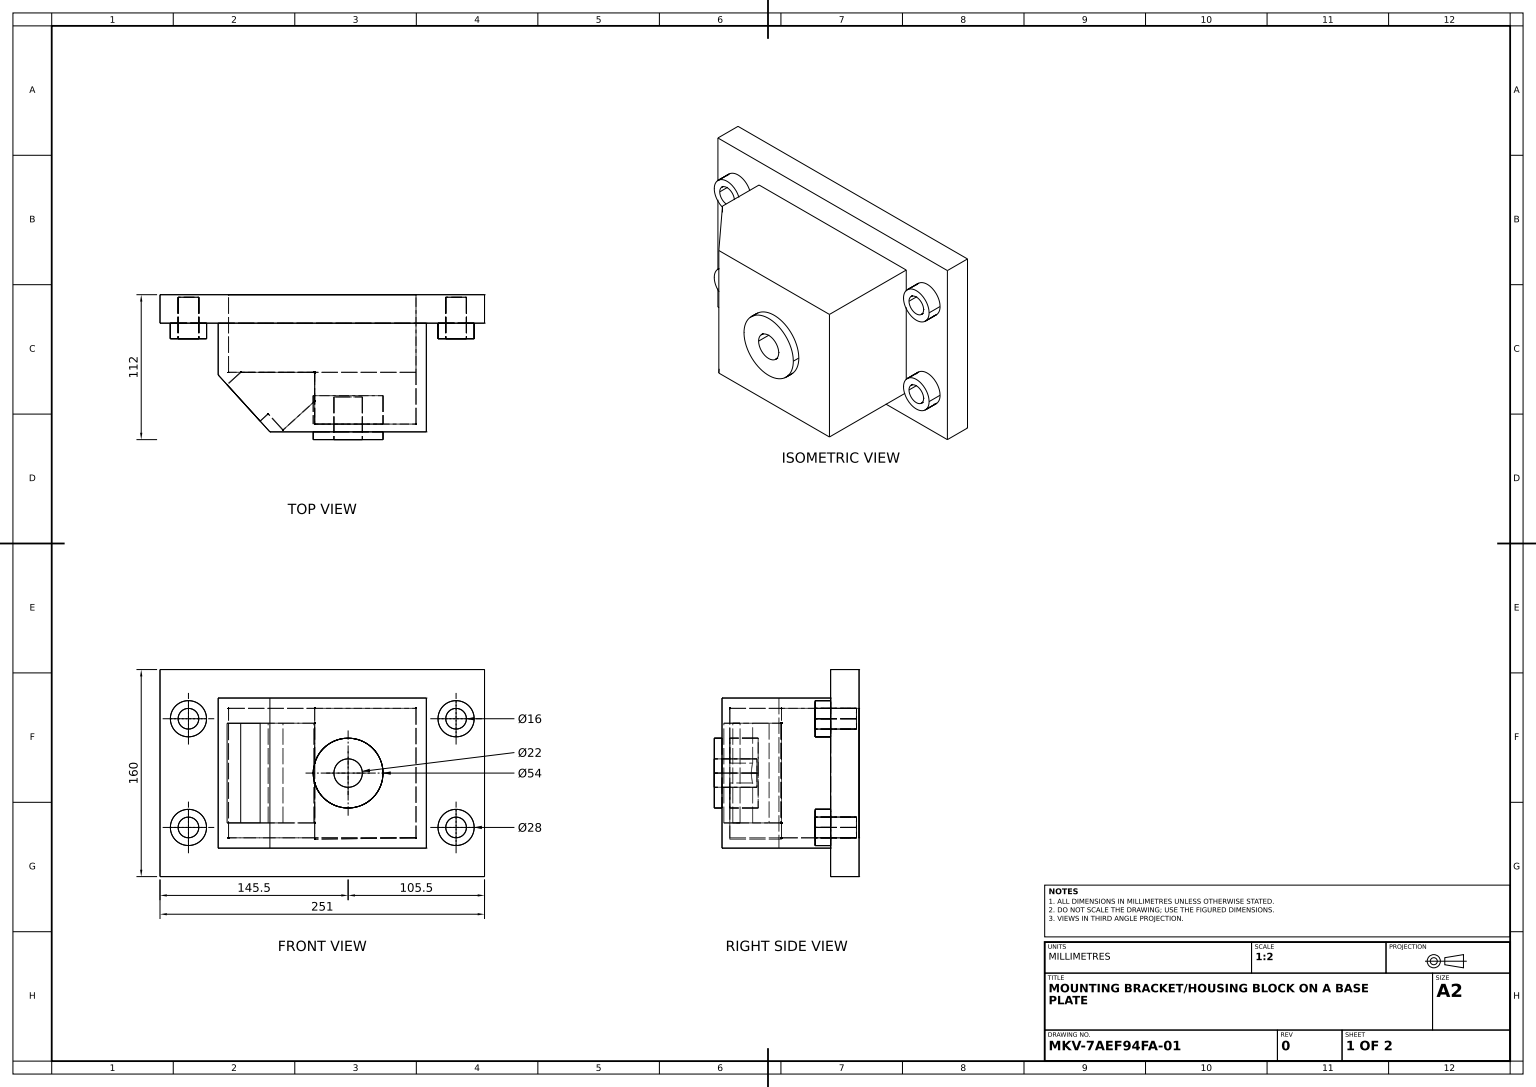
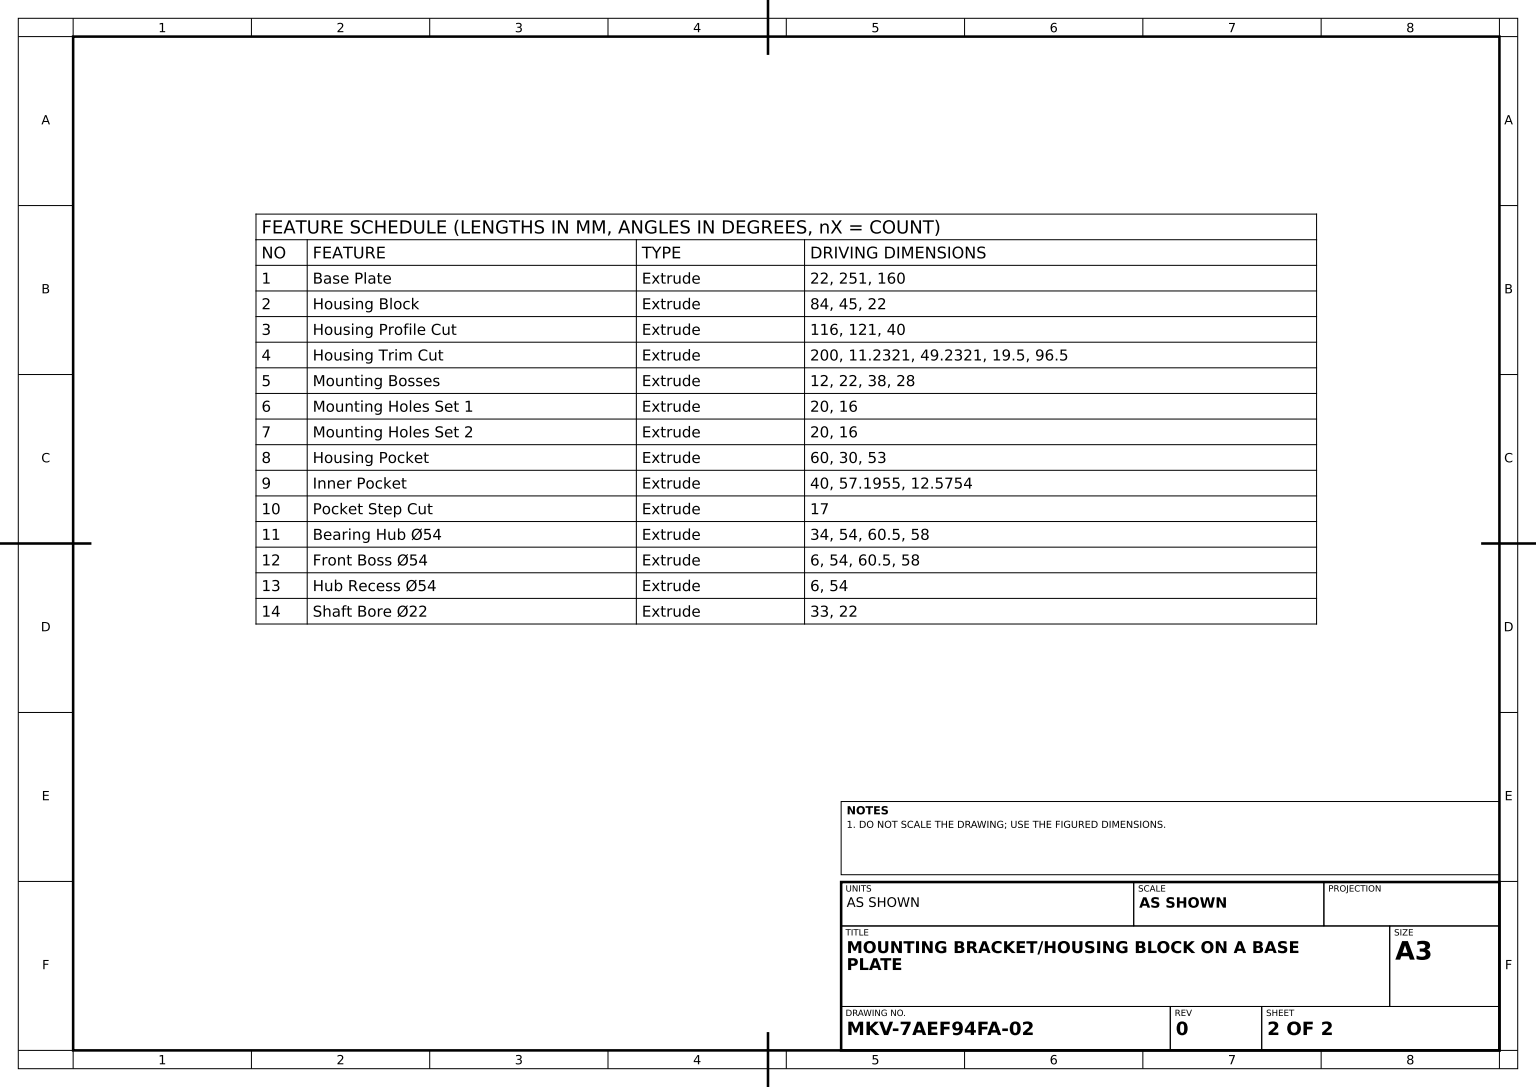
SolidWorks part; units mm, degrees
material "Plain Carbon Steel"
ref_plane "Front Plane" through (0, 0, 0) normal (0, 0, 1) x (1, 0, 0)
ref_plane "Top Plane" through (0, 0, 0) normal (0, 1, 0) x (1, 0, 0)
ref_plane "Right Plane" through (0, 0, 0) normal (1, 0, 0) x (0, 0, -1)
sketch "Base Plate Sketch" plane through (0, 0, 0) normal (0, 0, 1) x (1, 0, 0)
  line L0 (0, 0) -> (251, 0)
  line L1 (251, 0) -> (251, 160)
  line L2 (251, 160) -> (0, 160)
  line L3 (0, 160) -> (0, 0)
  dimension "D1" = 251
  dimension "D2" = 160
extrude "Base Plate" add sketch "Base Plate Sketch" along normal blind 22
sketch "Housing Block Sketch" plane through (0, 0, 22) normal (0, 0, 1) x (1, 0, 0)
  line L0 (251, 0) -> (251, 160) construction
  line L1 (45, 138) -> (206, 138)
  line L2 (45, 138) -> (45, 22)
  line L3 (45, 22) -> (206, 22)
  line L4 (206, 138) -> (206, 22)
  line L5 (0, 0) -> (251, 0) construction
  line L6 (251, 160) -> (0, 160) construction
  line L7 (0, 160) -> (0, 0) construction
  dimension "D1" = 45
  dimension "D2" = 22
  dimension "D3" = 22
  dimension "D4" = 45
extrude "Housing Block" add sketch "Housing Block Sketch" along normal blind 84
sketch "Housing Profile Cut Sketch" plane through (0, 22, 0) normal (0, -1, 0) x (1, 0, 0)
  line L0 (206, 106) -> (206, 22) construction
  line L1 (45, 106) -> (45, 22) construction
  line L2 (45, 22) -> (206, 22) construction
  line L3 (45, 106) -> (206, 106) construction
  line L4 (85, 106) -> (45, 62)
  line L5 (45, 106) -> (85, 106)
  line L6 (45, 62) -> (45, 106)
  dimension "D1" = 121
  dimension "D2" = 40
extrude "Housing Profile Cut" cut sketch "Housing Profile Cut Sketch" against normal blind 116
sketch "Housing Trim Cut Sketch" plane through (-6.2217, 0, 5.6561) normal (-0.7399, 0, 0.6727) x (0.6727, 0, 0.7399)
  line L0 (135.6108, 138) -> (135.6108, 22) construction
  line L5 (76.1466, 22) -> (135.6108, 22) construction
  line L11 (86.3787, 118.5) -> (86.3787, 41.5)
  line L14 (124.3787, 41.5) -> (124.3787, 118.5)
  line L16 (124.3787, 118.5) -> (86.3787, 118.5)
  line L18 (124.3787, 41.5) -> (86.3787, 41.5)
  line L19 (86.3787, 41.5) -> (86.3787, 118.5)
  dimension "D1" = 11.2321
  dimension "D2" = 49.2321
  dimension "D3" = 19.5
  dimension "D4" = 96.5
extrude "Housing Trim Cut" cut sketch "Housing Trim Cut Sketch" against normal blind 200 contours L18 L14 L16 L11
sketch "Mounting Bosses Sketch" plane through (0, 0, 22) normal (0, 0, 1) x (1, 0, 0)
  line L0 (251, 0) -> (251, 160) construction
  line L1 (0, 0) -> (251, 0) construction
  line L3 (251, 160) -> (0, 160) construction
  line L4 (0, 160) -> (0, 0) construction
  circle A0 centre (229, 122) radius 14
  circle A1 centre (229, 38) radius 14
  circle A2 centre (22, 38) radius 14
  circle A3 centre (22, 122) radius 14
  dimension "D1" = 28
  dimension "D2" = 28
  dimension "D3" = 28
  dimension "D4" = 28
  dimension "D10" = 28
  dimension "D11" = 28
  dimension "D12" = 28
  dimension "D13" = 28
  dimension "D5" = 22
  dimension "D6" = 22
  dimension "D7" = 38
  dimension "D8" = 38
  dimension "D9" = 84
  dimension "D14" = 22
  dimension "D15" = 38
  dimension "D16" = 22
  dimension "D17" = 38
extrude "Mounting Bosses" add sketch "Mounting Bosses Sketch" along normal blind 12
sketch "Mounting Holes Set 1 Sketch" plane through (0, 0, 22) normal (0, 0, 1) x (1, 0, 0)
  circle A0 centre (22, 122) radius 8
  circle A1 centre (22, 38) radius 8
  circle A2 centre (229, 38) radius 8
  circle A3 centre (229, 122) radius 8
  dimension "D1" = 16
  dimension "D2" = 16
  dimension "D3" = 16
  dimension "D4" = 16
  dimension "D5" = 16
extrude "Mounting Holes Set 1" cut sketch "Mounting Holes Set 1 Sketch" against normal blind 20
sketch "Mounting Holes Set 2 Sketch" plane through (0, 0, 34) normal (0, 0, 1) x (1, 0, 0)
  circle A0 centre (229, 122) radius 8
  circle A1 centre (229, 38) radius 8
  circle A2 centre (22, 38) radius 8
  circle A3 centre (22, 122) radius 8
  dimension "D1" = 16
  dimension "D2" = 16
  dimension "D3" = 16
  dimension "D4" = 16
  dimension "D5" = 16
extrude "Mounting Holes Set 2" cut sketch "Mounting Holes Set 2 Sketch" against normal blind 20
sketch "Housing Pocket Sketch" plane through (0, 0, 0) normal (0, 0, -1) x (-1, 0, 0)
  line L1 (-198, 130) -> (-53, 130)
  line L2 (-198, 130) -> (-198, 30)
  line L3 (-198, 30) -> (-53, 30)
  line L4 (-53, 130) -> (-53, 30)
  line L8 (-251, 160) -> (0, 160) construction
  line L9 (0, 0) -> (-251, 0) construction
  line L10 (0, 160) -> (0, 0) construction
  line L11 (-251, 0) -> (-251, 160) construction
  dimension "D1" = 30
  dimension "D2" = 30
  dimension "D3" = 53
  dimension "D4" = 53
extrude "Housing Pocket" cut sketch "Housing Pocket Sketch" against normal blind 60
sketch "Inner Pocket Sketch" plane through (0, 0, 60) normal (0, 0, -1) x (-1, 0, 0)
  line L0 (-198, 130) -> (-119.6067, 130)
  line L1 (-53, 130) -> (-198, 130) construction
  line L2 (-119.6067, 130) -> (-119.6067, 28.9246)
  line L3 (-119.6067, 28.9246) -> (-198, 30)
  line L4 (-198, 30) -> (-198, 130)
  line L5 (-62.4112, 118.5) -> (-62.4112, 41.5) construction
  line L6 (-118.9022, 41.5) -> (-62.4112, 41.5) construction
  dimension "D1" = 57.1955
  dimension "D2" = 12.5754
extrude "Inner Pocket" cut sketch "Inner Pocket Sketch" against normal blind 40
sketch "Pocket Step Cut Sketch" plane through (83.6662, 0, 92.0328) normal (-0.6727, 0, -0.7399) x (-0.7399, 0, 0.6727)
  line L0 (-47.6202, 118.5) -> (0, 118.5)
  line L1 (0, 160) -> (0, 0) construction
  line L2 (0, 118.5) -> (0, 41.5)
  line L3 (0, 41.5) -> (-47.6202, 41.5)
  line L4 (-47.6202, 41.5) -> (-47.6202, 118.5)
extrude "Pocket Step Cut" cut sketch "Pocket Step Cut Sketch" against normal blind 17
sketch "Bearing Hub Ø54 Sketch" plane through (0, 0, 106) normal (0, 0, 1) x (1, 0, 0)
  line L0 (85, 138) -> (85, 22) construction
  line L1 (85, 22) -> (206, 22) construction
  circle A0 centre (145.5, 80) radius 27
  dimension "D1" = 54
  dimension "D2" = 54
  dimension "D3" = 60.5
  dimension "D4" = 58
extrude "Bearing Hub Ø54" add sketch "Bearing Hub Ø54 Sketch" against normal blind 34
sketch "Front Boss Ø54 Sketch" plane through (0, 0, 106) normal (0, 0, 1) x (1, 0, 0)
  line L0 (85, 138) -> (85, 22) construction
  line L1 (85, 22) -> (206, 22) construction
  circle A0 centre (145.5, 80) radius 27
  dimension "D1" = 54
  dimension "D2" = 54
  dimension "D3" = 60.5
  dimension "D4" = 58
extrude "Front Boss Ø54" add sketch "Front Boss Ø54 Sketch" along normal blind 6
sketch "Hub Recess Ø54 Sketch" plane through (0, 0, 72) normal (0, 0, -1) x (-1, 0, 0)
  circle A0 centre (-145.5, 80) radius 27
  dimension "D1" = 54
  dimension "D2" = 54
extrude "Hub Recess Ø54" cut sketch "Hub Recess Ø54 Sketch" against normal blind 6
sketch "Shaft Bore Ø22 Sketch" plane through (0, 0, 112) normal (0, 0, 1) x (1, 0, 0)
  circle A0 centre (145.5, 80) radius 11
  dimension "D1" = 22
  dimension "D2" = 22
extrude "Shaft Bore Ø22" cut sketch "Shaft Bore Ø22 Sketch" against normal blind 33
